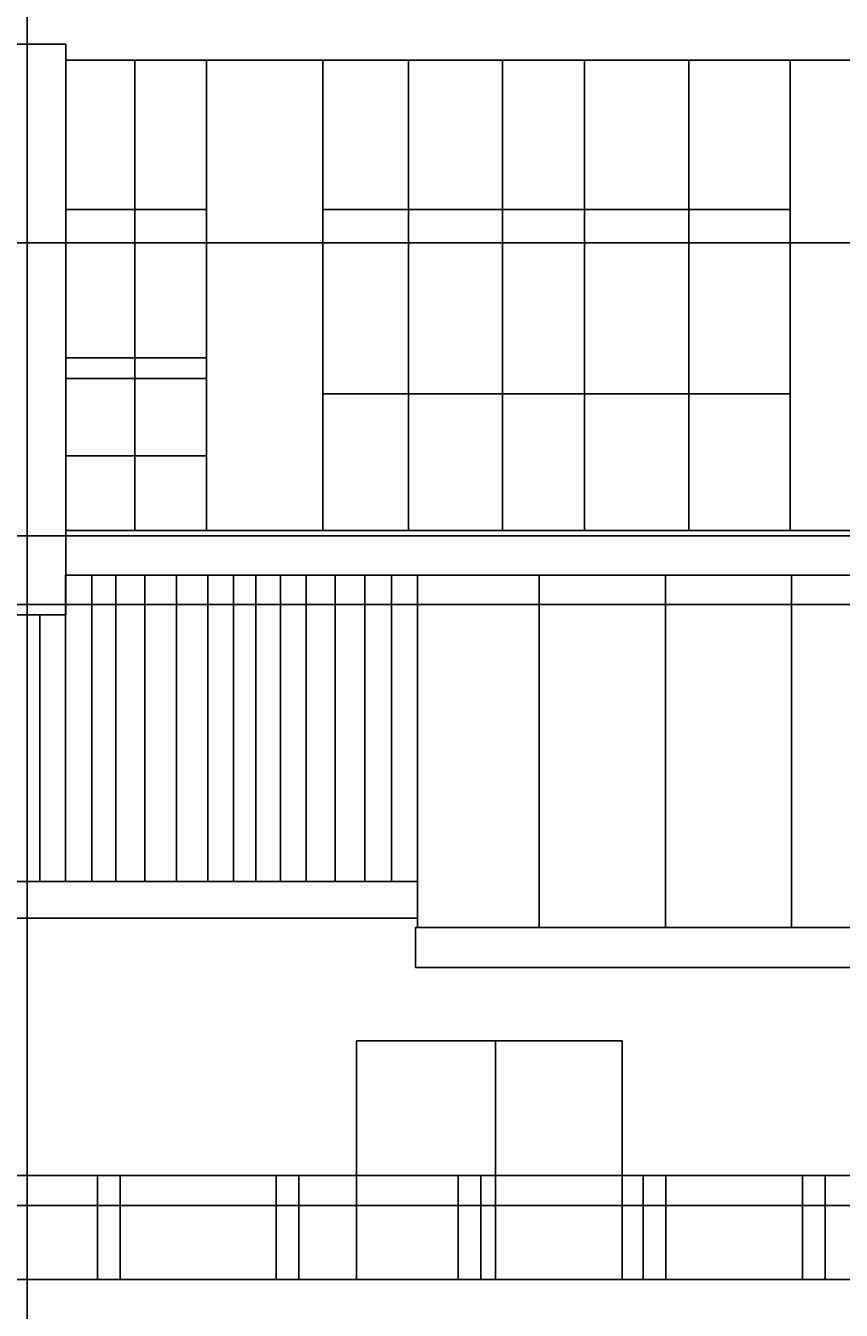
# Model space of a CAD drawing. Units: inches. Extents: x -117 to 121, y -77 to 40.
# Tile 25 of 45: x 28 to 50, y -43 to -8. Entities that reach past the tile are written whole.
import ezdxf

# ---------------------------------------------------------------- set-up
doc = ezdxf.new("R2010")
doc.units = ezdxf.units.IN
doc.header["$MEASUREMENT"] = 0
doc.layers.add('A-ANNO-DIMS', color=2, linetype='Continuous', lineweight=18)
doc.layers.add('A-ELEV', color=7, linetype='Continuous', lineweight=25)
doc.styles.get("Standard").update_dxf_attribs({"font": 'arial.ttf'})
doc.dimstyles.get("Standard").update_dxf_attribs({"dimtxt": 0.18, "dimasz": 0.18, "dimexe": 0.18, "dimexo": 0.0625, "dimgap": 0.09, "dimtad": 0, "dimtih": 1, "dimtoh": 1, "dimdec": 4, "dimzin": 0, "dimdsep": 46, "dimtxsty": 'Standard', "dimcen": 0.09, "dimadec": 0, "dimazin": 0, "dimtfac": 1, "dimtdec": 4, "dimtofl": 0, "dimtmove": 0, "dimatfit": 3, "dimfxl": 1, "dimtolj": 1, "dimtzin": 0, "dimarcsym": 0})

# ---------------------------------------------------------------- blocks, each defined once
blk = doc.blocks.new('*D49')
at = {"layer": 'A-ANNO-DIMS', "color": 0, "lineweight": -2, "transparency": 16777216}
for p, q in [((-45.422, -23.501), (120.84, -23.501)), ((120.66, -23.681), (120.66, -31.426)), ((120.66, -39.536), (120.66, -31.79)), ((-45.471, -39.716), (120.84, -39.716))]:
    blk.add_line(p, q, dxfattribs=at)
at = {"layer": 'A-ANNO-DIMS', "color": 0, "transparency": 16777216}
for points in [[(120.63, -23.681), (120.69, -23.681), (120.66, -23.501)], [(120.63, -39.536), (120.69, -39.536), (120.66, -39.716)]]:
    blk.add_solid(points, dxfattribs=at)
at = {"layer": 'Defpoints', "color": 0, "transparency": 16777216}
for p in [(-45.485, -23.501), (120.66, -23.501), (-45.533, -39.716)]:
    blk.add_point(p, dxfattribs=at)
at = {"layer": 'A-ANNO-DIMS', "color": 0, "transparency": 16777216, "insert": (120.66, -31.608), "char_height": 0.18, "attachment_point": 5}
blk.add_mtext('\\A1;16.215', dxfattribs=at)
blk = doc.blocks.new('*D50')
at = {"layer": 'A-ANNO-DIMS', "color": 0, "lineweight": -2, "transparency": 16777216}
for p, q in [((-47.458, -13.74), (120.84, -13.74)), ((120.66, -13.92), (120.66, -17.512)), ((120.66, -21.468), (120.66, -17.876)), ((-47.458, -21.648), (120.84, -21.648))]:
    blk.add_line(p, q, dxfattribs=at)
at = {"layer": 'A-ANNO-DIMS', "color": 0, "transparency": 16777216}
for points in [[(120.63, -13.92), (120.69, -13.92), (120.66, -13.74)], [(120.63, -21.468), (120.69, -21.468), (120.66, -21.648)]]:
    blk.add_solid(points, dxfattribs=at)
at = {"layer": 'Defpoints', "color": 0, "transparency": 16777216}
for p in [(-47.521, -13.74), (120.66, -13.74), (-47.521, -21.648)]:
    blk.add_point(p, dxfattribs=at)
at = {"layer": 'A-ANNO-DIMS', "color": 0, "transparency": 16777216, "insert": (120.66, -17.694), "char_height": 0.18, "attachment_point": 5}
blk.add_mtext('\\A1;7.908', dxfattribs=at)
blk = doc.blocks.new('*D53')
at = {"layer": 'A-ANNO-DIMS', "color": 0, "lineweight": -2, "transparency": 16777216}
for p, q in [((27.974, 10.841), (27.974, -77.193)), ((51.69, 10.9), (51.69, -77.193)), ((28.154, -77.013), (39.367, -77.013)), ((51.51, -77.013), (40.297, -77.013))]:
    blk.add_line(p, q, dxfattribs=at)
at = {"layer": 'A-ANNO-DIMS', "color": 0, "transparency": 16777216}
for points in [[(28.154, -76.983), (28.154, -77.043), (27.974, -77.013)], [(51.51, -76.983), (51.51, -77.043), (51.69, -77.013)]]:
    blk.add_solid(points, dxfattribs=at)
at = {"layer": 'Defpoints', "color": 0, "transparency": 16777216}
for p in [(27.974, 10.903), (51.69, 10.962), (51.69, -77.013)]:
    blk.add_point(p, dxfattribs=at)
at = {"layer": 'A-ANNO-DIMS', "color": 0, "transparency": 16777216, "insert": (39.832, -77.013), "char_height": 0.18, "attachment_point": 5}
blk.add_mtext('\\A1;23.716', dxfattribs=at)
blk = doc.blocks.new('*D58')
at = {"layer": 'A-ANNO-DIMS', "color": 0, "lineweight": -2, "transparency": 16777216}
for p, q in [((57.61, -7.947), (57.61, -77.193)), ((24.248, -8.105), (24.248, -77.193)), ((24.428, -77.013), (40.467, -77.013)), ((57.43, -77.013), (41.392, -77.013))]:
    blk.add_line(p, q, dxfattribs=at)
at = {"layer": 'A-ANNO-DIMS', "color": 0, "transparency": 16777216}
for points in [[(24.428, -76.983), (24.428, -77.043), (24.248, -77.013)], [(57.43, -76.983), (57.43, -77.043), (57.61, -77.013)]]:
    blk.add_solid(points, dxfattribs=at)
at = {"layer": 'Defpoints', "color": 0, "transparency": 16777216}
for p in [(57.61, -7.885), (24.248, -8.042), (57.61, -77.013)]:
    blk.add_point(p, dxfattribs=at)
at = {"layer": 'A-ANNO-DIMS', "color": 0, "transparency": 16777216, "insert": (40.929, -77.013), "char_height": 0.18, "attachment_point": 5}
blk.add_mtext('\\A1;33.362', dxfattribs=at)

msp = doc.modelspace()

# ---------------------------------------------------------------- linework, layer by layer
at = {"layer": 'A-ELEV'}
for p, q in [((29.012, -8.3785), (14.7397, -8.3785)), ((29.012, -23.7756), (29.012, -8.3785)), ((56.354, -8.8134), (29.012, -8.8134)), ((30.8752, -8.8134), (30.8752, -21.5025)), ((32.813, -8.8134), (32.813, -21.5025)), ((35.9521, -8.8134), (35.9521, -21.5025)), ((38.2591, -8.8134), (38.2591, -21.5025)), ((40.7968, -8.8134), (40.7968, -21.5025)), ((43.0114, -8.8134), (43.0114, -21.5025)), ((45.8259, -8.8134), (45.8259, -21.5025)), ((48.5665, -8.8134), (48.5665, -21.5025)), ((29.012, -12.8394), (32.813, -12.8394)), ((35.9521, -12.8394), (48.5665, -12.8394)), ((29.012, -16.8487), (32.813, -16.8487)), ((29.012, -17.4017), (32.813, -17.4017)), ((35.9521, -17.8165), (48.5665, -17.8165)), ((29.012, -19.4843), (32.813, -19.4843)), ((56.354, -21.5025), (29.012, -21.5025)), ((29.0053, -22.7074), (29.0053, -30.968)), ((56.4528, -22.7074), (29.012, -22.7074)), ((29.719, -22.7074), (29.719, -30.968)), ((30.3635, -22.7074), (30.3635, -30.968)), ((31.1462, -22.7074), (31.1462, -30.968)), ((31.998, -22.7074), (31.998, -30.968)), ((32.8497, -22.7074), (32.8497, -30.968)), ((33.5403, -22.7074), (33.5403, -30.968)), ((34.1388, -22.7074), (34.1388, -30.968)), ((34.8064, -22.7074), (34.8064, -30.968)), ((35.497, -22.7074), (35.497, -30.968)), ((36.2797, -22.7074), (36.2797, -30.968)), ((37.0854, -22.7074), (37.0854, -30.968)), ((37.7991, -22.7074), (37.7991, -30.968)), ((38.5013, -22.7074), (38.5013, -32.2104)), ((41.7888, -22.7074), (41.7888, -32.2104)), ((45.195, -22.7074), (45.195, -32.2104)), ((48.6012, -22.7074), (48.6012, -32.2104)), ((14.7397, -23.7756), (29.012, -23.7756)), ((28.3147, -23.7756), (28.3147, -30.968)), ((21.9795, -30.968), (38.5013, -30.968)), ((21.9795, -31.9617), (38.5013, -31.9617)), ((54.143, -32.2104), (38.4517, -32.2104)), ((38.4517, -32.2104), (38.4517, -33.2923)), ((38.4517, -33.2923), (54.143, -33.2923)), ((36.8562, -41.7053), (36.8562, -35.2709)), ((36.8562, -35.2709), (44.0284, -35.2709)), ((40.6078, -41.7053), (40.6078, -35.2709)), ((44.0284, -35.2709), (44.0284, -41.7053)), ((21.9795, -38.9022), (54.143, -38.9022)), ((29.8696, -41.7053), (29.8696, -38.9022)), ((30.4833, -41.7053), (30.4833, -38.9022)), ((34.6914, -41.7053), (34.6914, -38.9022)), ((35.3051, -41.7053), (35.3051, -38.9022)), ((39.6008, -41.7053), (39.6008, -38.9022)), ((40.2145, -41.7053), (40.2145, -38.9022)), ((44.5978, -41.7053), (44.5978, -38.9022)), ((45.2115, -41.7053), (45.2115, -38.9022)), ((48.8936, -41.7053), (48.8936, -38.9022)), ((49.5072, -41.7053), (49.5072, -38.9022)), ((37.6294, -41.7053), (21.9795, -41.7053)), ((68.508, -41.7053), (37.6294, -41.7053))]:
    msp.add_line(p, q, dxfattribs=at)

# ---------------------------------------------------------------- dimensions: what is measured, and where the dimension line sits
at = {"layer": 'A-ANNO-DIMS'}
for base, p1, p2, picture, middle in [((51.6901, -77.0135), (27.9744, 10.9032), (51.6901, 10.9623), '*D53', (39.8322, -77.0135)), ((57.6104, -77.0135), (24.2481, -8.0421), (57.6104, -7.8846), '*D58', (40.9293, -77.0135))]:
    dim = msp.add_linear_dim(base=base, p1=p1, p2=p2, dimstyle='Standard', override={"dimdec": 3, "dimlfac": 1, "dimrnd": 0, "dimzin": 0, "dimdsep": 46, "dimlunit": 2}, dxfattribs=at)
    dim.commit()
    dim.dimension.update_dxf_attribs({"geometry": picture, "text_midpoint": middle})
for base, p1, p2, picture, middle in [((120.6602, -13.74), (-47.5206, -21.6476), (-47.5206, -13.74), '*D50', (120.6602, -17.6938)), ((120.6602, -23.5007), (-45.5331, -39.716), (-45.4848, -23.5007), '*D49', (120.6602, -31.6083))]:
    dim = msp.add_linear_dim(base=base, p1=p1, p2=p2, angle=90, dimstyle='Standard', override={"dimdec": 3, "dimlfac": 1, "dimrnd": 0, "dimzin": 0, "dimdsep": 46, "dimlunit": 2}, dxfattribs=at)
    dim.commit()
    dim.dimension.update_dxf_attribs({"geometry": picture, "text_midpoint": middle})

doc.saveas('drawing.dxf')
